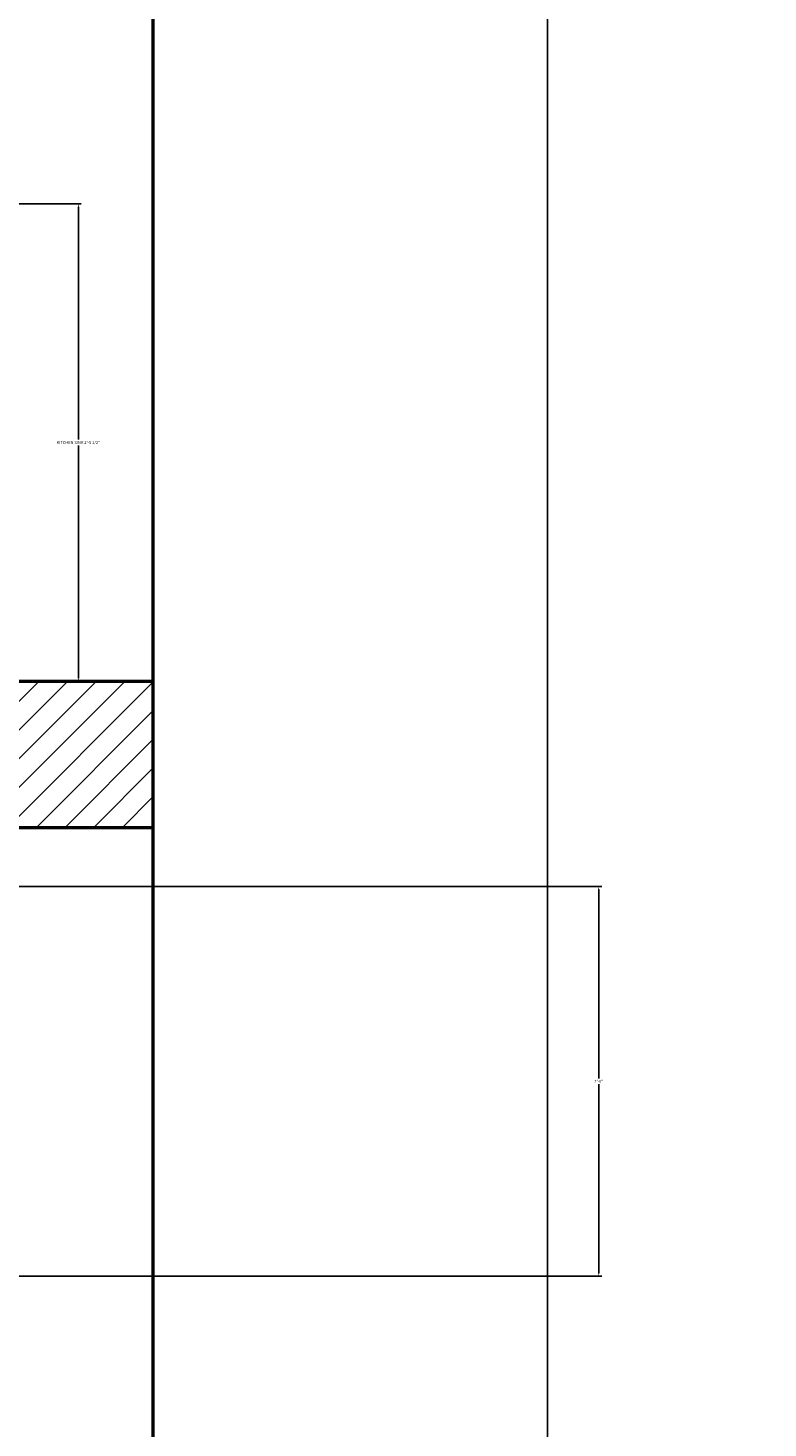
# Model space of a CAD drawing. Units: inches. Extents: x 0 to 281, y -535 to 46.
# Tile 13 of 22: x 236 to 281, y -168 to -82. Entities that reach past the tile are written whole.
import ezdxf

# ---------------------------------------------------------------- set-up
doc = ezdxf.new("R2010")
doc.units = ezdxf.units.IN
doc.header["$MEASUREMENT"] = 0
for name, color, linetype, lineweight in [('A-ANNO-DIMS', 2, 'Continuous', 18), ('A-COLS-PATT', 152, 'Continuous', 13), ('A-WALL', 7, 'Continuous', 50)]:
    doc.layers.add(name, color=color, linetype=linetype, lineweight=lineweight)
doc.styles.get("Standard").update_dxf_attribs({"font": 'arial.ttf'})
doc.dimstyles.get("Standard").update_dxf_attribs({"dimtxt": 0.18, "dimasz": 0.18, "dimexe": 0.18, "dimexo": 0.0625, "dimgap": 0.09, "dimtad": 0, "dimtih": 1, "dimtoh": 1, "dimdec": 0, "dimzin": 0, "dimdsep": 46, "dimlunit": 3, "dimtxsty": 'Standard', "dimcen": 0.09, "dimadec": 0, "dimazin": 0, "dimtfac": 1, "dimtdec": 0, "dimtofl": 0, "dimtmove": 0, "dimatfit": 3, "dimfxl": 1, "dimtolj": 1, "dimtzin": 0, "dimarcsym": 0})

# ---------------------------------------------------------------- blocks, each defined once
blk = doc.blocks.new('*D18')
at = {"layer": 'A-ANNO-DIMS', "color": 0, "lineweight": -2, "transparency": 16777216}
for p, q in [((243.521, 18.589), (267.926, 18.589)), ((267.746, 18.409), (267.746, -241.255)), ((267.746, -507.231), (267.746, -247.566)), ((243.521, -507.411), (267.926, -507.411))]:
    blk.add_line(p, q, dxfattribs=at)
at = {"layer": 'A-ANNO-DIMS', "color": 0, "transparency": 16777216}
for points in [[(267.716, 18.409), (267.776, 18.409), (267.746, 18.589)], [(267.716, -507.231), (267.776, -507.231), (267.746, -507.411)]]:
    blk.add_solid(points, dxfattribs=at)
at = {"layer": 'Defpoints', "color": 0, "transparency": 16777216}
for p in [(243.459, 18.589), (243.459, -507.411), (267.746, -507.411)]:
    blk.add_point(p, dxfattribs=at)
at = {"layer": 'A-ANNO-DIMS', "color": 0, "transparency": 16777216, "insert": (267.746, -244.411), "char_height": 6, "attachment_point": 5}
blk.add_mtext('\\A1;43\'-10"', dxfattribs=at)
blk = doc.blocks.new('*D30')
at = {"layer": 'A-ANNO-DIMS', "color": 0, "lineweight": -2, "transparency": 16777216}
for p, q in [((234.521, -93.018), (239.048, -93.018)), ((238.868, -93.198), (238.868, -107.531)), ((238.868, -122.231), (238.868, -107.897)), ((234.521, -122.411), (239.048, -122.411))]:
    blk.add_line(p, q, dxfattribs=at)
at = {"layer": 'A-ANNO-DIMS', "color": 0, "transparency": 16777216}
for points in [[(238.838, -93.198), (238.898, -93.198), (238.868, -93.018)], [(238.838, -122.231), (238.898, -122.231), (238.868, -122.411)]]:
    blk.add_solid(points, dxfattribs=at)
at = {"layer": 'Defpoints', "color": 0, "transparency": 16777216}
for p in [(234.459, -93.018), (234.459, -122.411), (238.868, -122.411)]:
    blk.add_point(p, dxfattribs=at)
at = {"layer": 'A-ANNO-DIMS', "color": 0, "transparency": 16777216, "insert": (238.868, -107.714), "char_height": 0.18, "attachment_point": 5}
blk.add_mtext('\\A1;KITCHEN SINK 2\'-5 1/2"', dxfattribs=at)
blk = doc.blocks.new('*D43')
at = {"layer": 'A-ANNO-DIMS', "color": 0, "lineweight": -2, "transparency": 16777216}
for p, q in [((93.521, -135.051), (271.089, -135.051)), ((270.909, -135.231), (270.909, -146.869)), ((270.909, -158.871), (270.909, -147.233)), ((93.521, -159.051), (271.089, -159.051))]:
    blk.add_line(p, q, dxfattribs=at)
at = {"layer": 'A-ANNO-DIMS', "color": 0, "transparency": 16777216}
for points in [[(270.879, -135.231), (270.939, -135.231), (270.909, -135.051)], [(270.879, -158.871), (270.939, -158.871), (270.909, -159.051)]]:
    blk.add_solid(points, dxfattribs=at)
at = {"layer": 'Defpoints', "color": 0, "transparency": 16777216}
for p in [(93.459, -135.051), (93.459, -159.051), (270.909, -159.051)]:
    blk.add_point(p, dxfattribs=at)
at = {"layer": 'A-ANNO-DIMS', "color": 0, "transparency": 16777216, "insert": (270.909, -147.051), "char_height": 0.18, "attachment_point": 5}
blk.add_mtext('\\A1;2\'-0"', dxfattribs=at)

msp = doc.modelspace()

# ---------------------------------------------------------------- hatches: boundary and pattern name
at = {"layer": 'A-COLS-PATT'}
h = msp.add_hatch(dxfattribs=at)
h.set_pattern_fill('ANSI31', color=256, scale=10)
h.paths.add_polyline_path([(36.459, 18.589), (27.459, 18.589), (27.459, 9.589), (36.459, 9.589)])
h.paths.add_polyline_path([(165.459, 18.589), (156.459, 18.589), (156.459, 9.589), (165.459, 9.589)])
h.paths.add_polyline_path([(243.459, 18.589), (234.459, 18.589), (234.459, 9.589), (243.459, 9.589)])
h.paths.add_polyline_path([(243.459, -122.411), (234.459, -122.411), (234.459, -131.411), (243.459, -131.411)])
h.paths.add_polyline_path([(36.459, -122.411), (27.459, -122.411), (27.459, -131.411), (36.459, -131.411)])
h.paths.add_polyline_path([(36.459, -498.411), (27.459, -498.411), (27.459, -507.411), (36.459, -507.411)])
h.paths.add_polyline_path([(243.459, -498.411), (234.459, -498.411), (234.459, -507.411), (243.459, -507.411)])
h.paths.add_polyline_path([(159.459, -498.411), (150.459, -498.411), (150.459, -507.411), (159.459, -507.411)])
h.paths.add_polyline_path([(36.459, -392.411), (27.459, -392.411), (27.459, -401.411), (36.459, -401.411)])
h.paths.add_polyline_path([(159.459, -392.411), (150.459, -392.411), (150.459, -401.411), (159.459, -401.411)])
h.paths.add_polyline_path([(243.459, -392.411), (234.459, -392.411), (234.459, -401.411), (243.459, -401.411)])
h.paths.add_polyline_path([(36.459, -263.411), (27.459, -263.411), (27.459, -272.411), (36.459, -272.411)])
h.paths.add_polyline_path([(243.459, -263.411), (234.459, -263.411), (234.459, -272.411), (243.459, -272.411)])

# ---------------------------------------------------------------- linework, layer by layer
at = {"layer": 'A-WALL'}
for p, q in [((243.459, 18.589), (243.459, -507.411)), ((189.459, -122.411), (243.459, -122.411)), ((189.459, -131.411), (243.459, -131.411))]:
    msp.add_line(p, q, dxfattribs=at)

# ---------------------------------------------------------------- dimensions: what is measured, and where the dimension line sits
at = {"layer": 'A-ANNO-DIMS'}
for base, p1, p2, override, picture, middle in [((267.746, -507.411), (243.459, 18.589), (243.459, -507.411), {"dimtxt": 6, "dimclrd": 0, "dimclre": 0, "dimclrt": 0}, '*D18', (267.746, -244.411)), ((270.909, -159.051), (93.459, -135.051), (93.459, -159.051), {"dimdec": 1, "dimlfac": 1, "dimrnd": 0, "dimzin": 1, "dimdsep": 46, "dimlunit": 4, "dimfrac": 2}, '*D43', (270.909, -147.051))]:
    dim = msp.add_linear_dim(base=base, p1=p1, p2=p2, angle=90, dimstyle='Standard', override=override, dxfattribs=at)
    dim.commit()
    dim.dimension.update_dxf_attribs({"geometry": picture, "text_midpoint": middle})
dim = msp.add_linear_dim(base=(238.868, -122.411), p1=(234.459, -93.018), p2=(234.459, -122.411), angle=270, text='KITCHEN SINK <>', dimstyle='Standard', override={"dimdec": 1, "dimlfac": 1, "dimrnd": 0, "dimzin": 1, "dimdsep": 46, "dimlunit": 4, "dimfrac": 2}, dxfattribs=at)
dim.commit()
dim.dimension.update_dxf_attribs({"geometry": '*D30', "text_midpoint": (238.868, -107.714)})

doc.saveas('drawing.dxf')
